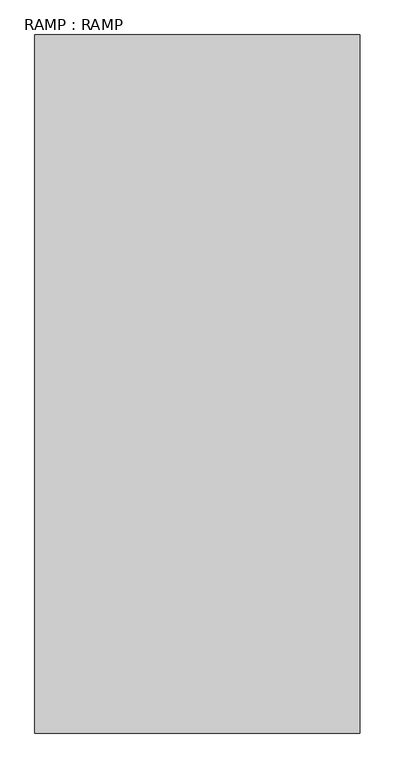
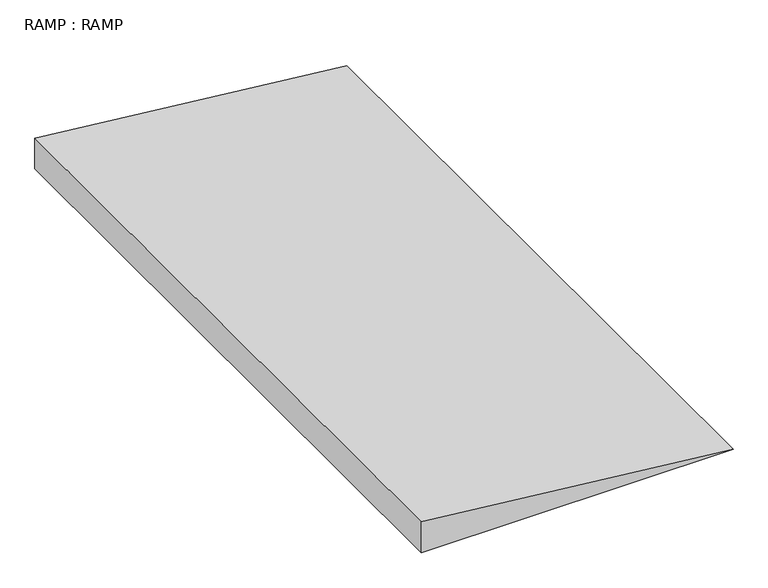
"""IFC4 building model written with IfcOpenShell, lengths in millimetres: proxy geometry, RAMP : RAMP."""

from ifc_helpers import new_model, si_unit, frame, origin, place, context, project, spatial, polyline, outline, extrude, source, transform, mapped, element, save


def ramp_ramp_f62ef563(model_context):
    return source(origin(), model_context, "Body", "SweptSolid", [
        extrude(outline(polyline([(-152.4, 1495.0722402), (-152.4, 3323.8722402), (37.3542959, 1495.0722402), (-152.4, 1495.0722402)])), frame((0.0, -4071.9657199, 0.0), z_axis=(0.0, 1.0, 0.0), x_axis=(0.0, 0.0, 1.0)), (0.0, 0.0, 1.0), 3924.3),
    ])


if __name__ == "__main__":
    model = new_model("IFC4")
    model_context = context("Model", 3, world=origin())
    ifc_project = project(units=[si_unit("LENGTHUNIT", "METRE", prefix="MILLI")], contexts=[model_context])
    site = spatial("IfcSite", under=ifc_project)
    building = spatial("IfcBuilding", under=site)
    placement = place(None, origin())
    ramp_ramp_shape = ramp_ramp_f62ef563(model_context)
    element("IfcBuildingElementProxy", 1, Name="RAMP : RAMP", ObjectType="RAMP : RAMP", at=placement, inside=building, context=model_context, shape_type="MappedRepresentation", body=[
        mapped(ramp_ramp_shape, transform((0.0, 0.0, 0.0), x_axis=(1.0, 0.0, 0.0), y_axis=(0.0, 1.0, 0.0), z_axis=(0.0, 0.0, 1.0))),
    ])
    save(model, "model.ifc")
